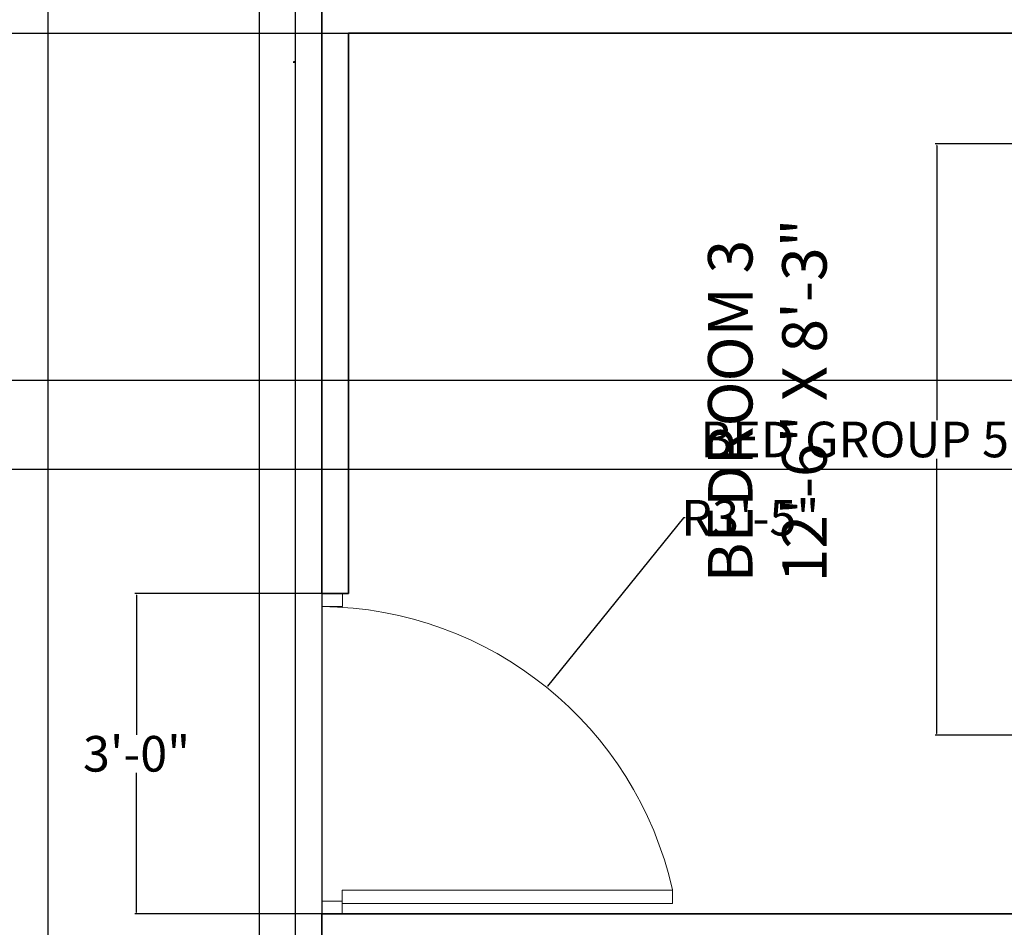
# Model space of a CAD drawing. Units: inches. Extents: x 311 to 754, y 60 to 497.
# Tile 7 of 11: x 530 to 641, y 194 to 296. Entities that reach past the tile are written whole.
import ezdxf

# ---------------------------------------------------------------- set-up
doc = ezdxf.new("R2010")
doc.units = ezdxf.units.IN
doc.header["$MEASUREMENT"] = 0
for name, color, linetype, lineweight in [('A-ANNO-DIMS', 2, 'Continuous', 18), ('A-AREA-IDEN', 1, 'Continuous', 18), ('A-WALL', 7, 'Continuous', 35), ('doors', 210, 'Continuous', 18)]:
    doc.layers.add(name, color=color, linetype=linetype, lineweight=lineweight)
doc.styles.get("Standard").update_dxf_attribs({"font": 'arial.ttf'})
doc.dimstyles.get("Standard").update_dxf_attribs({"dimtxt": 4, "dimasz": 0.18, "dimexe": 0.18, "dimexo": 0.0625, "dimgap": 0.09, "dimtad": 0, "dimtih": 1, "dimtoh": 1, "dimdec": 0, "dimrnd": 6, "dimzin": 0, "dimdsep": 46, "dimlunit": 3, "dimtxsty": 'Standard', "dimcen": 0.09, "dimadec": 0, "dimazin": 0, "dimtfac": 1, "dimtdec": 0, "dimtofl": 0, "dimtmove": 0, "dimatfit": 3, "dimfxl": 1, "dimtolj": 1, "dimtzin": 0, "dimarcsym": 0})

# ---------------------------------------------------------------- blocks, each defined once
blk = doc.blocks.new('*D108')
at = {"layer": 'A-ANNO-DIMS', "color": 0, "lineweight": -2, "transparency": 16777216}
for p, q in [((642.81, 281.79), (632.73, 281.79)), ((632.91, 281.61), (632.91, 250.72)), ((632.91, 215.5), (632.91, 246.4)), ((642.81, 215.32), (632.73, 215.32))]:
    blk.add_line(p, q, dxfattribs=at)
at = {"layer": 'A-ANNO-DIMS', "color": 0, "transparency": 16777216}
for points in [[(632.88, 281.61), (632.94, 281.61), (632.91, 281.79)], [(632.88, 215.5), (632.94, 215.5), (632.91, 215.32)]]:
    blk.add_solid(points, dxfattribs=at)
at = {"layer": 'Defpoints', "color": 0, "transparency": 16777216}
for p in [(642.88, 281.79), (632.91, 215.32), (642.88, 215.32)]:
    blk.add_point(p, dxfattribs=at)
at = {"layer": 'A-ANNO-DIMS', "color": 0, "transparency": 16777216, "insert": (632.91, 248.56), "char_height": 4, "attachment_point": 5}
blk.add_mtext('\\A1;BED GROUP 5\'-6 1/2"', dxfattribs=at)
blk = doc.blocks.new('*D131')
at = {"layer": 'A-ANNO-DIMS', "color": 0, "lineweight": -2, "transparency": 16777216}
for p, q in [((563.74, 231.24), (542.82, 231.24)), ((543, 231.06), (543, 215.37)), ((543, 195.42), (543, 211.1)), ((563.74, 195.24), (542.82, 195.24))]:
    blk.add_line(p, q, dxfattribs=at)
at = {"layer": 'A-ANNO-DIMS', "color": 0, "transparency": 16777216}
for points in [[(542.97, 231.06), (543.03, 231.06), (543, 231.24)], [(542.97, 195.42), (543.03, 195.42), (543, 195.24)]]:
    blk.add_solid(points, dxfattribs=at)
at = {"layer": 'Defpoints', "color": 0, "transparency": 16777216}
for p in [(543, 231.24), (563.8, 231.24), (563.8, 195.24)]:
    blk.add_point(p, dxfattribs=at)
at = {"layer": 'A-ANNO-DIMS', "color": 0, "transparency": 16777216, "insert": (543, 213.24), "char_height": 4, "attachment_point": 5}
blk.add_mtext('\\A1;3\'-0"', dxfattribs=at)
blk = doc.blocks.new('*D132')
at = {"layer": 'A-ANNO-DIMS', "color": 0, "lineweight": -2, "transparency": 16777216}
for p, q in [((526.91, 339.18), (526.91, 66.26)), ((560.82, 339.18), (560.82, 66.26)), ((527.09, 66.44), (536.87, 66.44)), ((560.64, 66.44), (550.86, 66.44))]:
    blk.add_line(p, q, dxfattribs=at)
at = {"layer": 'A-ANNO-DIMS', "color": 0, "transparency": 16777216}
for points in [[(527.09, 66.47), (527.09, 66.41), (526.91, 66.44)], [(560.64, 66.47), (560.64, 66.41), (560.82, 66.44)]]:
    blk.add_solid(points, dxfattribs=at)
at = {"layer": 'Defpoints', "color": 0, "transparency": 16777216}
for p in [(526.91, 339.24), (560.82, 339.24), (526.91, 66.44)]:
    blk.add_point(p, dxfattribs=at)
at = {"layer": 'A-ANNO-DIMS', "color": 0, "transparency": 16777216, "insert": (543.87, 66.44), "char_height": 4, "attachment_point": 5}
blk.add_mtext('\\A1;2\'-10"', dxfattribs=at)
blk = doc.blocks.new('*D134')
at = {"layer": 'A-ANNO-DIMS', "color": 0, "lineweight": -2, "transparency": 16777216}
for p, q in [((494.8, 342.18), (494.8, 66.26)), ((563.8, 342.18), (563.8, 66.26)), ((494.98, 66.44), (523.9, 66.44)), ((563.62, 66.44), (534.71, 66.44))]:
    blk.add_line(p, q, dxfattribs=at)
at = {"layer": 'A-ANNO-DIMS', "color": 0, "transparency": 16777216}
for points in [[(494.98, 66.47), (494.98, 66.41), (494.8, 66.44)], [(563.62, 66.47), (563.62, 66.41), (563.8, 66.44)]]:
    blk.add_solid(points, dxfattribs=at)
at = {"layer": 'Defpoints', "color": 0, "transparency": 16777216}
for p in [(494.8, 342.24), (563.8, 342.24), (563.8, 66.44)]:
    blk.add_point(p, dxfattribs=at)
at = {"layer": 'A-ANNO-DIMS', "color": 0, "transparency": 16777216, "insert": (529.3, 66.44), "char_height": 4, "attachment_point": 5}
blk.add_mtext('\\A1;5\'-9"', dxfattribs=at)
blk = doc.blocks.new('*D139')
at = {"layer": 'A-ANNO-DIMS', "color": 0, "lineweight": -2, "transparency": 16777216}
for p, q in [((449.87, 255.24), (743.78, 255.24)), ((743.6, 255.06), (743.6, 252.37)), ((743.6, 245.42), (743.6, 248.11)), ((449.87, 245.24), (743.78, 245.24))]:
    blk.add_line(p, q, dxfattribs=at)
at = {"layer": 'A-ANNO-DIMS', "color": 0, "transparency": 16777216}
for points in [[(743.57, 255.06), (743.63, 255.06), (743.6, 255.24)], [(743.57, 245.42), (743.63, 245.42), (743.6, 245.24)]]:
    blk.add_solid(points, dxfattribs=at)
at = {"layer": 'Defpoints', "color": 0, "transparency": 16777216}
for p in [(449.8, 255.24), (743.6, 255.24), (449.8, 245.24)]:
    blk.add_point(p, dxfattribs=at)
at = {"layer": 'A-ANNO-DIMS', "color": 0, "transparency": 16777216, "insert": (743.6, 250.24), "char_height": 4, "attachment_point": 5}
blk.add_mtext('\\A1;0\'-10"', dxfattribs=at)
blk = doc.blocks.new('*D140')
at = {"layer": 'A-ANNO-DIMS', "color": 0, "lineweight": -2, "transparency": 16777216}
for p, q in [((449.87, 294.24), (743.78, 294.24)), ((743.6, 294.06), (743.6, 276.87)), ((743.6, 255.42), (743.6, 272.6)), ((449.87, 255.24), (743.78, 255.24))]:
    blk.add_line(p, q, dxfattribs=at)
at = {"layer": 'A-ANNO-DIMS', "color": 0, "transparency": 16777216}
for points in [[(743.57, 294.06), (743.63, 294.06), (743.6, 294.24)], [(743.57, 255.42), (743.63, 255.42), (743.6, 255.24)]]:
    blk.add_solid(points, dxfattribs=at)
at = {"layer": 'Defpoints', "color": 0, "transparency": 16777216}
for p in [(449.8, 294.24), (743.6, 294.24), (449.8, 255.24)]:
    blk.add_point(p, dxfattribs=at)
at = {"layer": 'A-ANNO-DIMS', "color": 0, "transparency": 16777216, "insert": (743.6, 274.74), "char_height": 4, "attachment_point": 5}
blk.add_mtext('\\A1;3\'-3"', dxfattribs=at)
blk = doc.blocks.new('*D146')
at = {"layer": 'A-ANNO-DIMS', "color": 0, "lineweight": -2, "transparency": 16777216}
for p, q in [((533.04, 385.85), (533.04, 66.26)), ((556.78, 385.85), (556.78, 66.26)), ((533.22, 66.44), (533.47, 66.44)), ((556.6, 66.44), (556.34, 66.44))]:
    blk.add_line(p, q, dxfattribs=at)
at = {"layer": 'A-ANNO-DIMS', "color": 0, "transparency": 16777216}
for points in [[(533.22, 66.47), (533.22, 66.41), (533.04, 66.44)], [(556.6, 66.47), (556.6, 66.41), (556.78, 66.44)]]:
    blk.add_solid(points, dxfattribs=at)
at = {"layer": 'Defpoints', "color": 0, "transparency": 16777216}
for p in [(533.04, 385.92), (556.78, 385.92), (556.78, 66.44)]:
    blk.add_point(p, dxfattribs=at)
at = {"layer": 'A-ANNO-DIMS', "color": 0, "transparency": 16777216, "insert": (544.91, 66.44), "char_height": 4, "attachment_point": 5}
blk.add_mtext('\\A1;1\'-11 1/2"', dxfattribs=at)
blk = doc.blocks.new('*D154')
at = {"layer": 'A-ANNO-DIMS', "color": 0, "lineweight": -2, "transparency": 16777216}
for p, q in [((603.74, 340.99), (587.72, 322.37)), ((603.92, 340.99), (603.74, 340.99)), ((560.7, 290.89), (560.7, 291.07)), ((560.61, 290.98), (560.79, 290.98))]:
    blk.add_line(p, q, dxfattribs=at)
at = {"layer": 'A-ANNO-DIMS', "color": 0, "transparency": 16777216}
blk.add_solid([(587.69, 322.39), (587.74, 322.35), (587.6, 322.23)], dxfattribs=at)
at = {"layer": 'Defpoints', "color": 0, "transparency": 16777216}
for p in [(587.6, 322.23), (560.7, 290.98)]:
    blk.add_point(p, dxfattribs=at)
at = {"layer": 'A-ANNO-DIMS', "color": 0, "transparency": 16777216, "insert": (611.24, 340.99), "char_height": 4, "attachment_point": 5}
blk.add_mtext('\\A1;R3\'-5"', dxfattribs=at)
blk = doc.blocks.new('*D156')
at = {"layer": 'A-ANNO-DIMS', "color": 0, "lineweight": -2, "transparency": 16777216}
for p, q in [((604.46, 239.76), (589.17, 220.85)), ((604.64, 239.76), (604.46, 239.76)), ((563.31, 188.97), (563.49, 188.97)), ((563.4, 188.88), (563.4, 189.06))]:
    blk.add_line(p, q, dxfattribs=at)
at = {"layer": 'A-ANNO-DIMS', "color": 0, "transparency": 16777216}
blk.add_solid([(589.15, 220.87), (589.2, 220.83), (589.06, 220.71)], dxfattribs=at)
at = {"layer": 'Defpoints', "color": 0, "transparency": 16777216}
for p in [(589.06, 220.71), (563.4, 188.97)]:
    blk.add_point(p, dxfattribs=at)
at = {"layer": 'A-ANNO-DIMS', "color": 0, "transparency": 16777216, "insert": (611.96, 239.76), "char_height": 4, "attachment_point": 5}
blk.add_mtext('\\A1;R3\'-5"', dxfattribs=at)

msp = doc.modelspace()

# ---------------------------------------------------------------- linework, layer by layer
at = {"layer": 'A-WALL'}
for p, q in [((563.8, 231.24), (563.8, 297.24)), ((713.8, 294.24), (566.8, 294.24)), ((566.8, 231.24), (566.8, 294.24)), ((566.8, 231.24), (563.8, 231.24)), ((563.8, 192.24), (563.8, 195.24)), ((713.8, 195.24), (563.8, 195.24))]:
    msp.add_line(p, q, dxfattribs=at)
at = {"layer": 'doors'}
for points in [[(566.13, 229.78), (566.13, 231.23), (563.82, 231.23), (563.82, 229.78)], [(566.11, 197.93), (566.11, 196.41), (603.23, 196.41), (603.23, 197.93)], [(563.8, 195.24), (563.8, 196.68), (566.11, 196.68), (566.11, 195.24)]]:
    msp.add_lwpolyline(points, close=True, dxfattribs=at)
msp.add_arc((563.4, 188.97), 40.82, 12.6904, 89.4184, dxfattribs=at)

# ---------------------------------------------------------------- texts
at = {"layer": 'A-AREA-IDEN', "ltscale": 50, "insert": (607.21, 232.5), "char_height": 5, "attachment_point": 1, "rotation": 90}
msp.add_mtext_dynamic_manual_height_columns('BEDROOM 3\\P12\'-6" X 8\'-3"\\P ', width=51.3734, gutter_width=1, heights=[0], dxfattribs=at)

# ---------------------------------------------------------------- dimensions: what is measured, and where the dimension line sits
at = {"layer": 'A-ANNO-DIMS'}
for base, p1, p2, picture, middle in [((556.78, 66.44), (533.04, 385.92), (556.78, 385.92), '*D146', (544.91, 66.44)), ((563.8, 66.44), (494.8, 342.24), (563.8, 342.24), '*D134', (529.3, 66.44)), ((526.91, 66.44), (560.82, 339.24), (526.91, 339.24), '*D132', (543.87, 66.44))]:
    dim = msp.add_linear_dim(base=base, p1=p1, p2=p2, dimstyle='Standard', override={"dimdec": 1, "dimlfac": 1, "dimrnd": 0, "dimzin": 1, "dimdsep": 46, "dimlunit": 4, "dimfrac": 2}, dxfattribs=at)
    dim.commit()
    dim.dimension.update_dxf_attribs({"geometry": picture, "text_midpoint": middle})
for center, mpoint, picture, middle in [((560.7, 290.98), (587.6, 322.23), '*D154', (611.24, 340.99)), ((563.4, 188.97), (589.06, 220.71), '*D156', (611.96, 239.76))]:
    dim = msp.add_radius_dim(center=center, mpoint=mpoint, dimstyle='Standard', override={"dimdec": 1, "dimlfac": 1, "dimrnd": 0, "dimzin": 1, "dimdsep": 46, "dimlunit": 4, "dimfrac": 2}, dxfattribs=at)
    dim.commit()
    dim.dimension.update_dxf_attribs({"geometry": picture, "text_midpoint": middle, "dimtype": 164})
for base, p1, p2, picture, middle in [((743.6, 294.24), (449.8, 255.24), (449.8, 294.24), '*D140', (743.6, 274.74)), ((743.6, 255.24), (449.8, 245.24), (449.8, 255.24), '*D139', (743.6, 250.24)), ((543, 231.24), (563.8, 195.24), (563.8, 231.24), '*D131', (543, 213.24))]:
    dim = msp.add_linear_dim(base=base, p1=p1, p2=p2, angle=90, dimstyle='Standard', override={"dimdec": 1, "dimlfac": 1, "dimrnd": 0, "dimzin": 1, "dimdsep": 46, "dimlunit": 4, "dimfrac": 2}, dxfattribs=at)
    dim.commit()
    dim.dimension.update_dxf_attribs({"geometry": picture, "text_midpoint": middle})
dim = msp.add_linear_dim(base=(632.91, 215.32), p1=(642.88, 281.79), p2=(642.88, 215.32), angle=270, text='BED GROUP <>', dimstyle='Standard', override={"dimdec": 1, "dimlfac": 1, "dimrnd": 0, "dimzin": 1, "dimdsep": 46, "dimlunit": 4, "dimfrac": 2}, dxfattribs=at)
dim.commit()
dim.dimension.update_dxf_attribs({"geometry": '*D108', "text_midpoint": (632.91, 248.56)})

doc.saveas('drawing.dxf')
